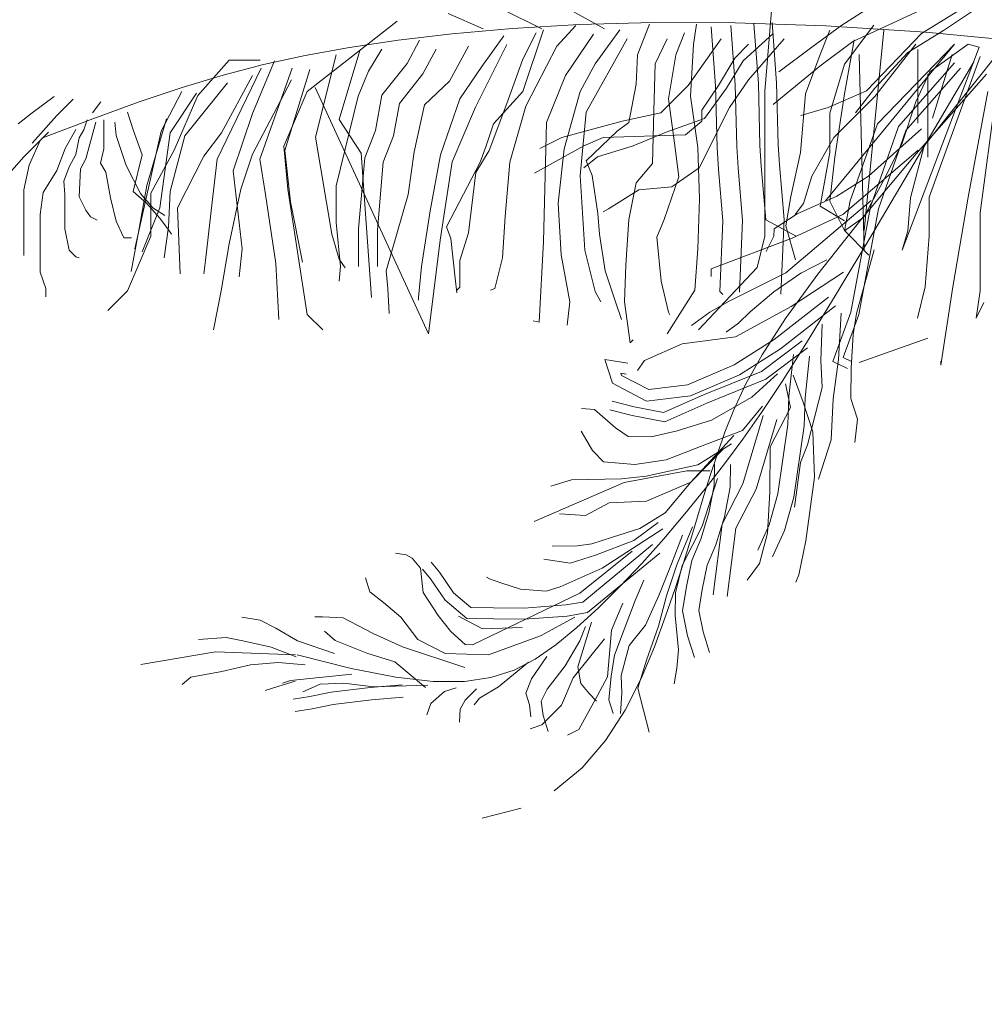
# Model space of a CAD drawing. Units: millimetres. Extents: x 595116 to 630915, y 909473 to 920225.
# Tile 82 of 134: x 629711.176 to 629720.161, y 919266.512 to 919275.684. Entities that reach past the tile are written whole.
import ezdxf

# ---------------------------------------------------------------- set-up
doc = ezdxf.new("R2010")
doc.units = ezdxf.units.MM
doc.layers.add('Dimension', color=3, linetype='Continuous', lineweight=18)
doc.layers.add('L-PLNT', color=85, linetype='Continuous', lineweight=13)
doc.styles.get("Standard").update_dxf_attribs({"font": 'arial.ttf'})
doc.dimstyles.new('ISO-25', dxfattribs={"dimtxt": 9, "dimasz": 6, "dimexe": 1.25, "dimexo": 0.625, "dimtad": 1, "dimlunit": 4, "dimtxsty": 'Standard', "dimcen": 2.5, "dimadec": 0, "dimazin": 0, "dimtfac": 1, "dimtmove": 0, "dimatfit": 3, "dimfxl": 1, "dimarcsym": 0})

# ---------------------------------------------------------------- blocks, each defined once
blk = doc.blocks.new('A$C4FB75ABC')
for p, q in [((2.1065, 2.3741), (2.087, 2.1315)), ((2.5983, 2.3508), (2.4757, 2.2759)), ((1.3881, 2.2867), (1.3008, 2.3255)), ((1.5337, 2.2867), (1.4367, 2.3352)), ((1.6891, 2.2867), (1.6017, 2.3352)), ((2.2781, 2.2963), (2.353, 2.344)), ((2.3054, 2.2555), (2.4825, 2.3372)), ((2.6119, 2.3372), (2.5302, 2.2827)), ((1.1746, 2.3061), (0.9513, 2.1315)), ((1.6258, 2.2976), (1.4598, 2.2878)), ((1.8099, 2.3026), (1.6258, 2.2976)), ((1.8004, 2.299), (1.7712, 2.2224)), ((2.0136, 2.3019), (1.8099, 2.3026)), ((1.9171, 2.299), (1.9098, 2.248)), ((2.2382, 2.2942), (2.0136, 2.3019)), ((2.0597, 2.2997), (2.0708, 2.1511)), ((2.1047, 2.3031), (2.1159, 2.1533)), ((1.3106, 2.2744), (1.1767, 2.2586)), ((1.4598, 2.2878), (1.3106, 2.2744)), ((1.5376, 2.2844), (1.4866, 2.1313)), ((1.5194, 2.2771), (1.4866, 2.2115)), ((1.6179, 2.2954), (1.5705, 2.2443)), ((1.6617, 2.2735), (1.5924, 2.1714)), ((1.7274, 2.2844), (1.6654, 2.2006)), ((1.8879, 2.2771), (1.8661, 2.2224)), ((1.9536, 2.2917), (1.9646, 2.1459)), ((2.0023, 2.2954), (2.0134, 2.1483)), ((2.1078, 2.2759), (2.0328, 2.2078)), ((2.2032, 2.2419), (2.2781, 2.2963)), ((2.2482, 2.2839), (2.2239, 2.2232)), ((2.4852, 2.2785), (2.2382, 2.2942)), ((2.3575, 2.296), (2.2846, 2.199)), ((2.3818, 2.2839), (2.3332, 1.7863)), ((2.4757, 2.2759), (2.3394, 2.1329)), ((2.5302, 2.2827), (2.4416, 2.2282)), ((2.7559, 2.2536), (2.4852, 2.2785)), ((1.1767, 2.2586), (1.0564, 2.241)), ((1.23, 2.2589), (1.1992, 2.2008)), ((1.4391, 2.2699), (1.3844, 2.1933)), ((1.7456, 2.2626), (1.6435, 2.0802)), ((1.8442, 2.2626), (1.815, 2.2006)), ((1.9783, 2.2623), (1.8966, 2.1465)), ((2.0124, 2.2146), (2.0465, 2.2487)), ((2.135, 2.2623), (2.0465, 2.1602)), ((2.2236, 2.1942), (2.3054, 2.2555)), ((2.5574, 2.2487), (2.2372, 1.8605)), ((2.3089, 2.2596), (2.2846, 2.1261)), ((2.462, 2.2487), (2.3599, 2.1193)), ((2.3667, 2.0512), (2.5574, 2.2487)), ((2.6937, 2.2623), (2.4825, 1.9967)), ((2.5915, 2.2487), (2.4961, 2.1806)), ((2.6187, 2.2419), (2.5915, 2.2487)), ((1.0564, 2.241), (0.9464, 2.2213)), ((1.0815, 2.2334), (1.0304, 2.062)), ((1.1363, 2.237), (1.1034, 2.1823)), ((1.2713, 2.237), (1.2384, 2.175)), ((1.3515, 2.2443), (1.3041, 2.1568)), ((1.4464, 2.2479), (1.3687, 2.0927)), ((1.5705, 2.2443), (1.4939, 2.0948)), ((1.9098, 2.248), (1.9025, 2.1203)), ((2.1214, 2.1806), (2.2032, 2.2419)), ((2.4416, 2.2282), (2.3599, 2.1397)), ((2.428, 1.738), (2.6187, 2.2419)), ((2.4668, 2.2354), (2.4668, 2.0533)), ((0.7572, 2.2091), (0.6795, 2.1218)), ((0.8348, 2.2091), (0.7572, 2.2091)), ((0.8699, 2.2079), (0.8151, 2.0766)), ((0.9464, 2.2213), (0.8429, 2.1986)), ((1.0231, 2.2224), (0.972, 2.0182)), ((1.1992, 2.2008), (1.1362, 2.1221)), ((1.4866, 2.2115), (1.4464, 2.1021)), ((1.6654, 2.2006), (1.6289, 2.1313)), ((1.7712, 2.2224), (1.7675, 2.1495)), ((1.815, 2.2006), (1.8113, 2.0838)), ((1.8661, 2.2224), (1.8478, 2.113)), ((1.9715, 2.1465), (2.0124, 2.2146)), ((2.0328, 2.2078), (1.992, 2.1397)), ((2.2239, 2.2232), (2.1875, 2.1261)), ((2.3211, 2.2232), (2.3332, 1.7378)), ((2.5572, 2.203), (2.4187, 2.0449)), ((2.6056, 2.2048), (2.4676, 1.9701)), ((2.6209, 2.2188), (2.4948, 1.8695)), ((2.5518, 2.2232), (2.5032, 2.0655)), ((0.837, 2.1896), (0.7276, 1.9635)), ((0.8429, 2.1986), (0.7422, 2.1723)), ((0.9137, 2.1896), (0.8334, 1.9635)), ((0.9575, 2.186), (0.8954, 1.9854)), ((1.1034, 2.1823), (1.0779, 2.1203)), ((1.2384, 2.175), (1.18, 2.1021)), ((1.3844, 2.1933), (1.3297, 2.113)), ((2.1078, 2.0989), (2.2236, 2.1942)), ((2.2846, 2.199), (2.2482, 2.0776)), ((2.5724, 2.1897), (2.4365, 2.0345)), ((2.4961, 2.1806), (2.462, 2.1057)), ((0.7422, 2.1723), (0.6405, 2.1416)), ((0.7531, 2.1531), (0.6473, 2.0218)), ((0.8151, 2.1714), (0.7385, 2.0291)), ((0.9125, 2.1606), (0.8154, 1.9763)), ((1.3041, 2.1568), (1.2421, 2.0984)), ((1.5924, 2.1714), (1.5449, 2.0547)), ((2.0465, 2.1602), (1.9988, 2.0921)), ((2.0708, 2.1511), (2.0745, 1.9975)), ((2.1159, 2.1533), (2.1196, 1.9995)), ((2.6368, 2.1742), (2.4628, 1.9766)), ((2.4911, 2.1747), (2.4911, 1.9684)), ((0.6405, 2.1416), (0.5342, 2.1057)), ((0.64, 2.1313), (0.5889, 2.0328)), ((0.6765, 2.1276), (0.6108, 2.0291)), ((0.9513, 2.1315), (0.8931, 1.9957)), ((1.2522, 1.53), (0.9707, 2.1412)), ((1.4866, 2.1313), (1.4136, 2.051)), ((1.6289, 2.1313), (1.5887, 1.989)), ((1.7675, 2.1495), (1.7493, 2.0547)), ((1.8966, 2.1465), (1.8285, 2.0784)), ((1.9306, 2.0852), (1.9715, 2.1465)), ((1.992, 2.1397), (1.9375, 2.0648)), ((1.9646, 2.1459), (1.9682, 1.9927)), ((2.0134, 2.1483), (2.017, 1.9949)), ((2.087, 2.1315), (2.087, 1.7725)), ((2.1875, 2.1261), (2.1754, 1.9805)), ((2.3394, 2.1329), (2.244, 2.0921)), ((2.2846, 2.1261), (2.2604, 1.9684)), ((2.3599, 2.1397), (2.3122, 2.0784)), ((2.6404, 2.1315), (2.5918, 1.8695)), ((0.2683, 2.0784), (0.3228, 2.1193)), ((0.3296, 2.0716), (0.3705, 2.1125)), ((0.4182, 2.0784), (0.4386, 2.1057)), ((0.5342, 2.1057), (0.4195, 2.0639)), ((0.6795, 2.1218), (0.6213, 1.986)), ((1.0779, 2.1203), (1.0231, 1.8978)), ((1.1362, 2.1221), (1.1203, 2.0346)), ((1.18, 2.1021), (1.1654, 2.0218)), ((1.3297, 2.113), (1.2822, 1.9744)), ((1.4464, 2.1021), (1.4026, 1.9854)), ((1.8478, 2.113), (1.8624, 2.0036)), ((1.9025, 2.1203), (1.9208, 1.9927)), ((2.3599, 2.1193), (2.2577, 2.0172)), ((2.462, 2.1057), (2.428, 2.0035)), ((2.6598, 2.1218), (2.6209, 1.8307)), ((0.2342, 2.0512), (0.2683, 2.0784)), ((0.505, 2.0802), (0.5196, 2.0364)), ((1.2421, 2.0984), (1.2165, 1.9817)), ((1.3687, 2.0927), (1.3105, 1.9569)), ((1.4939, 2.0948), (1.4537, 1.9562)), ((1.6435, 2.0802), (1.6289, 1.9234)), ((1.8285, 2.0784), (1.7331, 2.058)), ((1.8113, 2.0838), (1.8077, 1.9526)), ((1.9988, 2.0921), (1.9238, 1.9422)), ((1.9306, 2.058), (1.9306, 2.0852)), ((2.244, 2.0921), (2.1759, 2.0716)), ((2.2482, 2.0776), (2.2482, 1.9805)), ((0.2683, 2.0035), (0.3296, 2.0716)), ((0.4195, 2.0639), (0.2927, 2.0154)), ((0.4049, 2.0609), (0.3966, 2.0361)), ((0.427, 2.0554), (0.4021, 1.9643)), ((0.4463, 2.0609), (0.4463, 1.9892)), ((0.4739, 2.0554), (0.4767, 2.0223)), ((0.6018, 2.0636), (0.5533, 1.8986)), ((0.8151, 2.0766), (0.7677, 1.9343)), ((1.0304, 2.062), (1.0852, 1.9781)), ((1.5449, 2.0547), (1.5376, 1.7593)), ((1.7331, 2.058), (1.5832, 2.0172)), ((1.7493, 2.0547), (1.7201, 2.0328)), ((1.9375, 2.0648), (1.8421, 2.0308)), ((1.8898, 2.024), (1.9306, 2.058)), ((0.3092, 2.0308), (0.2479, 1.9695)), ((0.3773, 2.0376), (0.3501, 1.9899)), ((0.3966, 2.0361), (0.3855, 2.0168)), ((0.5196, 2.0364), (0.5415, 1.9744)), ((0.5889, 2.0328), (0.5232, 1.741)), ((0.6108, 2.0291), (0.5853, 1.8431)), ((0.7385, 2.0291), (0.6947, 1.9708)), ((1.1203, 2.0346), (1.0939, 1.9669)), ((1.4136, 2.051), (1.3953, 1.9963)), ((1.7201, 2.0328), (1.6435, 1.9598)), ((1.8421, 2.0308), (1.7603, 1.9967)), ((2.2985, 1.8605), (2.3667, 2.0512)), ((2.4756, 2.0387), (2.3438, 1.9217)), ((2.4187, 2.0449), (2.3489, 1.8456)), ((2.4365, 2.0345), (2.3686, 1.8404)), ((0.2887, 2.0103), (0.2615, 1.9491)), ((0.3855, 2.0168), (0.3773, 1.9754)), ((0.4767, 2.0223), (0.5015, 1.9478)), ((0.6473, 2.0218), (0.6108, 1.8833)), ((0.972, 2.0182), (1.0122, 1.7775)), ((1.1654, 2.0218), (1.1399, 1.9562)), ((1.5832, 2.0172), (1.5287, 1.9899)), ((1.6377, 1.9967), (1.6854, 2.0172)), ((1.6854, 2.0172), (1.8898, 2.024)), ((2.2577, 2.0172), (2.2032, 1.9218)), ((0.3501, 1.9899), (0.3296, 1.9354)), ((0.4463, 1.9892), (0.438, 1.9533)), ((0.6213, 1.986), (0.563, 1.8792)), ((0.8931, 1.9957), (0.9028, 1.8889)), ((0.8954, 1.9854), (0.91, 1.8577)), ((1.2165, 1.9817), (1.2019, 1.876)), ((1.4026, 1.9854), (1.3698, 1.9307)), ((1.3953, 1.9963), (1.3807, 1.9562)), ((1.5151, 1.9286), (1.6377, 1.9967)), ((1.5887, 1.989), (1.5741, 1.8541)), ((1.7603, 1.9967), (1.6718, 1.9695)), ((1.8624, 2.0036), (1.8734, 1.9197)), ((1.9208, 1.9927), (1.9244, 1.865)), ((1.9682, 1.9927), (1.9719, 1.938)), ((2.017, 1.9949), (2.0206, 1.9417)), ((2.0745, 1.9975), (2.0779, 1.946)), ((2.1196, 1.9995), (2.1229, 1.9495)), ((2.1754, 1.9805), (2.1511, 1.8713)), ((2.2482, 1.9805), (2.2239, 1.847)), ((2.4673, 1.986), (2.2802, 1.8264)), ((2.428, 2.0035), (2.3871, 1.9218)), ((2.4825, 1.9967), (2.4484, 1.8673)), ((0.2479, 1.9695), (0.2002, 1.915)), ((0.3773, 1.9754), (0.3607, 1.945)), ((0.4021, 1.9643), (0.3883, 1.9395)), ((0.5415, 1.9744), (0.5196, 1.8833)), ((0.6947, 1.9708), (0.629, 1.8431)), ((0.7276, 1.9635), (0.713, 1.8358)), ((0.8154, 1.9763), (0.7863, 1.8889)), ((0.8334, 1.9635), (0.848, 1.876)), ((1.0939, 1.9669), (1.0786, 1.7905)), ((1.0852, 1.9781), (1.1107, 1.6207)), ((1.1399, 1.9562), (1.1253, 1.7884)), ((1.2822, 1.9744), (1.2567, 1.8358)), ((1.3105, 1.9569), (1.2814, 1.7628)), ((1.3807, 1.9562), (1.2968, 1.7957)), ((1.4537, 1.9562), (1.4428, 1.8213)), ((1.6718, 1.9695), (1.6377, 1.9422)), ((1.6435, 1.9598), (1.6581, 1.9234)), ((2.2604, 1.9684), (2.2482, 1.8591)), ((2.4628, 1.9766), (2.3249, 1.8127)), ((2.4676, 1.9701), (2.3552, 1.7802)), ((0.2615, 1.9491), (0.2479, 1.8878)), ((0.3296, 1.9354), (0.2956, 1.881)), ((0.3607, 1.945), (0.3469, 1.9091)), ((0.3883, 1.9395), (0.3855, 1.8705)), ((0.438, 1.9533), (0.4518, 1.9312)), ((0.4518, 1.9312), (0.4629, 1.8677)), ((0.5015, 1.9478), (0.5374, 1.8788)), ((0.7677, 1.9343), (0.7896, 1.741)), ((1.3698, 1.9307), (1.3515, 1.7811)), ((1.8077, 1.9526), (1.7675, 1.9051)), ((1.9238, 1.9422), (1.8557, 1.8946)), ((1.9719, 1.938), (1.9828, 1.8103)), ((2.0206, 1.9417), (2.0317, 1.8114)), ((2.0779, 1.946), (2.0893, 1.8127)), ((2.1229, 1.9495), (2.1345, 1.8136)), ((0.3469, 1.9091), (0.3497, 1.876)), ((1.6289, 1.9234), (1.6398, 1.7374)), ((1.6581, 1.9234), (1.6727, 1.8285)), ((1.8734, 1.9197), (1.8369, 1.814)), ((2.2032, 1.9218), (2.1827, 1.8537)), ((2.3438, 1.9217), (2.2657, 1.8718)), ((2.3871, 1.9218), (2.3326, 1.8197)), ((0.2479, 1.8878), (0.2479, 1.8061)), ((0.5196, 1.8833), (0.5524, 1.8541)), ((0.5533, 1.8986), (0.5339, 1.7919)), ((0.6108, 1.8833), (0.6072, 1.7957)), ((0.7863, 1.8889), (0.7572, 1.7531)), ((0.9028, 1.8889), (0.9513, 1.5785)), ((1.0231, 1.8978), (1.0231, 1.8067)), ((1.7739, 1.8878), (1.699, 1.8401)), ((1.7675, 1.9051), (1.7493, 1.814)), ((1.8557, 1.8946), (1.7739, 1.8878)), ((0.2956, 1.881), (0.2887, 1.8265)), ((0.3497, 1.876), (0.3497, 1.8512)), ((0.3855, 1.8705), (0.4021, 1.8374)), ((0.4629, 1.8677), (0.4767, 1.8098)), ((0.5374, 1.8788), (0.5678, 1.8429)), ((0.563, 1.8792), (0.563, 1.7725)), ((0.848, 1.876), (0.8735, 1.7045)), ((0.91, 1.8577), (0.9392, 1.7082)), ((1.2019, 1.876), (1.1472, 1.6863)), ((1.9244, 1.865), (1.9208, 1.741)), ((2.3505, 1.8613), (2.1386, 1.6813)), ((2.1511, 1.8713), (2.1389, 1.7985)), ((2.2657, 1.8718), (2.167, 1.8279)), ((2.2482, 1.8591), (2.2846, 1.7863)), ((2.2849, 1.7856), (2.2985, 1.8605)), ((2.4484, 1.8673), (2.4416, 1.7856)), ((2.4948, 1.8695), (2.4948, 1.7725)), ((2.5918, 1.8695), (2.553, 1.6464)), ((0.3497, 1.8512), (0.3497, 1.7904)), ((0.4021, 1.8374), (0.4132, 1.8208)), ((0.5853, 1.8431), (0.5415, 1.7337)), ((0.5524, 1.8541), (0.5853, 1.8176)), ((0.5678, 1.8429), (0.5982, 1.8236)), ((0.629, 1.8431), (0.6363, 1.679)), ((0.713, 1.8358), (0.6984, 1.7118)), ((1.2567, 1.8358), (1.2348, 1.6973)), ((1.5741, 1.8541), (1.5814, 1.7264)), ((1.699, 1.8401), (1.6854, 1.8333)), ((2.1827, 1.8537), (2.1623, 1.8265)), ((2.2239, 1.847), (2.2846, 1.8106)), ((2.3489, 1.8456), (2.3004, 1.5838)), ((2.3686, 1.8404), (2.32, 1.5785)), ((0.2887, 1.8265), (0.2887, 1.7516)), ((0.4132, 1.8208), (0.4297, 1.8125)), ((0.4767, 1.8098), (0.496, 1.7684)), ((0.5853, 1.8176), (0.6072, 1.7884)), ((1.4428, 1.8213), (1.4355, 1.7191)), ((1.6727, 1.8285), (1.6763, 1.7775)), ((1.7493, 1.814), (1.742, 1.7009)), ((1.8369, 1.814), (1.8186, 1.7702)), ((1.9828, 1.8103), (1.9755, 1.6352)), ((2.0317, 1.8114), (2.0243, 1.6332)), ((2.0893, 1.8127), (2.1647, 1.7725)), ((2.167, 1.8279), (2.1099, 1.791)), ((2.1345, 1.8136), (2.1268, 1.6289)), ((2.2802, 1.8264), (2.1549, 1.7678)), ((2.3249, 1.8127), (2.2184, 1.678)), ((2.3326, 1.8197), (2.2849, 1.7856)), ((2.6209, 1.8307), (2.6209, 1.6367)), ((0.2479, 1.8061), (0.2479, 1.7448)), ((0.3497, 1.7904), (0.3607, 1.738)), ((0.5339, 1.7919), (0.5145, 1.6852)), ((0.6072, 1.7957), (0.5962, 1.7191)), ((0.6072, 1.7884), (0.6144, 1.7775)), ((1.0231, 1.8067), (1.0341, 1.6973)), ((1.0786, 1.7905), (1.0786, 1.6973)), ((1.1253, 1.7884), (1.1253, 1.7665)), ((1.2968, 1.7957), (1.3078, 1.7665)), ((2.1099, 1.791), (2.1096, 1.7722)), ((2.1389, 1.7985), (2.1632, 1.7135)), ((2.2846, 1.7863), (2.3453, 1.7256)), ((2.4416, 1.7856), (2.428, 1.738)), ((0.496, 1.7684), (0.5153, 1.7684)), ((0.563, 1.7725), (0.5048, 1.6367)), ((1.0122, 1.7775), (1.0304, 1.7155)), ((1.1253, 1.7665), (1.1253, 1.7301)), ((1.2814, 1.7628), (1.2522, 1.53)), ((1.3078, 1.7665), (1.3187, 1.6681)), ((1.3515, 1.7811), (1.3297, 1.7118)), ((1.6763, 1.7775), (1.6909, 1.6863)), ((1.8186, 1.7702), (1.8296, 1.6608)), ((2.1549, 1.7678), (1.9538, 1.6913)), ((2.087, 1.7725), (2.0676, 1.6949)), ((2.1096, 1.7722), (2.0903, 1.7347)), ((2.3552, 1.7802), (2.2641, 1.6283)), ((2.4948, 1.7725), (2.485, 1.6464)), ((0.2479, 1.7448), (0.2479, 1.7243)), ((0.2887, 1.7516), (0.2887, 1.6835)), ((0.3607, 1.738), (0.3773, 1.7214)), ((0.7572, 1.7531), (0.7377, 1.6367)), ((0.7896, 1.741), (0.7823, 1.6717)), ((1.5376, 1.7593), (1.5267, 1.5587)), ((1.6398, 1.7374), (1.6654, 1.6352)), ((1.9208, 1.741), (1.9135, 1.6389)), ((2.3582, 1.7386), (2.3145, 1.5808)), ((0.3773, 1.7214), (0.3855, 1.7187)), ((0.6984, 1.7118), (0.6947, 1.679)), ((1.0304, 1.7155), (1.045, 1.6936)), ((1.1253, 1.7301), (1.1253, 1.6973)), ((1.3297, 1.7118), (1.3297, 1.6462)), ((1.4355, 1.7191), (1.4172, 1.6425)), ((1.5814, 1.7264), (1.6033, 1.6097)), ((2.2409, 1.7138), (2.1763, 1.6807)), ((0.8735, 1.7045), (0.8808, 1.566)), ((1.0341, 1.6973), (1.0304, 1.6608)), ((1.1472, 1.6863), (1.1509, 1.6425)), ((1.2348, 1.6973), (1.2275, 1.6207)), ((1.6909, 1.6863), (1.7164, 1.6097)), ((1.742, 1.7009), (1.7383, 1.6097)), ((2.0676, 1.6949), (1.922, 1.5397)), ((1.9538, 1.6913), (1.9536, 1.6725)), ((0.2887, 1.6835), (0.3024, 1.6426)), ((1.3187, 1.6681), (1.3224, 1.6316)), ((2.1386, 1.6813), (1.998, 1.6115)), ((2.1763, 1.6807), (2.1096, 1.6345)), ((2.2184, 1.678), (2.1385, 1.568)), ((2.2819, 1.6831), (2.1525, 1.5981)), ((0.3024, 1.6426), (0.3024, 1.6222)), ((1.1509, 1.6425), (1.1545, 1.5805)), ((1.3297, 1.6462), (1.3224, 1.6389)), ((1.4172, 1.6425), (1.4063, 1.6389)), ((1.8296, 1.6608), (1.8478, 1.5842)), ((1.9135, 1.6389), (1.8444, 1.53)), ((2.485, 1.6464), (2.4656, 1.5688)), ((2.553, 1.6464), (2.5239, 1.4523)), ((0.5048, 1.6367), (0.4562, 1.5882)), ((0.7377, 1.6367), (0.7183, 1.5397)), ((1.2275, 1.6207), (1.2275, 1.6134)), ((1.6654, 1.6352), (1.68, 1.6097)), ((1.9755, 1.6352), (1.9828, 1.628)), ((2.1096, 1.6345), (2.0504, 1.5844)), ((2.2452, 1.6213), (2.1098, 1.5157)), ((2.2641, 1.6283), (2.1904, 1.5079)), ((2.6209, 1.6367), (2.6112, 1.5688)), ((1.6033, 1.6097), (1.596, 1.5514)), ((1.7164, 1.6097), (1.731, 1.566)), ((1.7383, 1.6097), (1.7529, 1.5076)), ((1.998, 1.6115), (1.9504, 1.5839)), ((2.1525, 1.5981), (2.0137, 1.5227)), ((2.2623, 1.5995), (2.1258, 1.493)), ((2.6112, 1.5688), (2.6307, 1.6076)), ((0.9513, 1.5785), (0.9901, 1.5397)), ((1.8478, 1.5842), (1.8515, 1.5769)), ((1.9504, 1.5839), (1.9047, 1.5506)), ((2.0504, 1.5844), (2.0217, 1.5565)), ((2.1385, 1.568), (2.0803, 1.4783)), ((2.3004, 1.5838), (2.256, 1.4617)), ((2.2767, 1.5813), (2.2695, 1.4664)), ((2.32, 1.5785), (2.2812, 1.4717)), ((2.3145, 1.5808), (2.3062, 1.5281)), ((1.5267, 1.5587), (1.5121, 1.5623)), ((2.0217, 1.5565), (1.9912, 1.5343)), ((2.2292, 1.5537), (2.2261, 1.4651)), ((2.0137, 1.5227), (1.8814, 1.5056)), ((2.1098, 1.5157), (2.0109, 1.453)), ((2.3062, 1.5281), (2.3013, 1.4452)), ((2.4911, 1.5193), (2.3211, 1.4586)), ((1.7529, 1.5076), (1.7602, 1.5149)), ((1.8814, 1.5056), (1.7884, 1.4636)), ((2.1258, 1.493), (2.0238, 1.4284)), ((2.1796, 1.5129), (2.0785, 1.437)), ((2.1927, 1.4954), (2.0894, 1.4177)), ((2.1904, 1.5079), (2.1298, 1.4122)), ((1.7084, 1.4073), (1.6895, 1.4666)), ((1.6895, 1.4666), (1.747, 1.4576)), ((2.0803, 1.4783), (2.039, 1.4043)), ((2.1578, 1.4791), (2.1468, 1.3743)), ((2.1979, 1.4749), (2.187, 1.3714)), ((2.2695, 1.4664), (2.2568, 1.3685)), ((2.2812, 1.4717), (2.3006, 1.462)), ((1.7884, 1.4636), (1.7711, 1.4393)), ((2.0109, 1.453), (1.8951, 1.4036)), ((2.2261, 1.4651), (2.2289, 1.3972)), ((2.256, 1.4617), (2.2916, 1.4439)), ((2.3013, 1.4452), (2.3002, 1.3698)), ((2.5239, 1.4523), (2.5239, 1.462)), ((1.7313, 1.4266), (1.7295, 1.4323)), ((1.7295, 1.4323), (1.7427, 1.4302)), ((1.7987, 1.3918), (1.7313, 1.4266)), ((2.0238, 1.4284), (1.9024, 1.3766)), ((2.0785, 1.437), (1.9344, 1.3786)), ((2.0894, 1.4177), (1.9429, 1.3584)), ((2.1181, 1.4308), (2.055, 1.3732)), ((2.1569, 1.4277), (2.1816, 1.3609)), ((1.7936, 1.3632), (1.7084, 1.4073)), ((1.8951, 1.4036), (1.7987, 1.3918)), ((2.039, 1.4043), (2.0098, 1.3416)), ((2.1298, 1.4122), (2.0784, 1.3347)), ((2.1385, 1.406), (2.1509, 1.3473)), ((2.2289, 1.3972), (2.1929, 1.2544)), ((1.9024, 1.3766), (1.7936, 1.3632)), ((1.9344, 1.3786), (1.8357, 1.3347)), ((2.055, 1.3732), (1.9542, 1.3161)), ((2.1468, 1.3743), (2.1439, 1.3053)), ((2.187, 1.3714), (2.1842, 1.3016)), ((2.2568, 1.3685), (2.2516, 1.2668)), ((2.3002, 1.3698), (2.3165, 1.3187)), ((1.6641, 1.3427), (1.6321, 1.345)), ((1.7623, 1.3489), (1.7078, 1.3628)), ((1.8357, 1.3347), (1.7623, 1.3489)), ((1.9429, 1.3584), (1.8383, 1.3119)), ((2.0811, 1.3502), (2.0312, 1.2905)), ((2.1509, 1.3473), (2.1005, 1.25)), ((2.1816, 1.3609), (2.2062, 1.287)), ((1.7163, 1.2967), (1.6641, 1.3427)), ((1.7575, 1.3275), (1.7024, 1.3416)), ((1.8383, 1.3119), (1.7575, 1.3275)), ((2.0098, 1.3416), (1.9878, 1.2857)), ((2.0784, 1.3347), (2.0319, 1.2687)), ((2.0829, 1.3276), (2.0324, 1.158)), ((1.7481, 1.2755), (1.7163, 1.2967)), ((1.9542, 1.3161), (1.869, 1.289)), ((2.1165, 1.3176), (2.065, 1.1449)), ((2.1439, 1.3053), (2.1195, 1.1332)), ((2.1842, 1.3016), (2.1591, 1.1247)), ((2.3165, 1.3187), (2.31, 1.2603)), ((1.6589, 1.2409), (1.6313, 1.2885)), ((1.8046, 1.2748), (1.7481, 1.2755)), ((1.869, 1.289), (1.8046, 1.2748)), ((2.0103, 1.2776), (1.903, 1.1622)), ((2.0312, 1.2905), (1.9421, 1.2559)), ((1.9878, 1.2857), (1.9691, 1.2327)), ((2.2062, 1.287), (2.2097, 1.1745)), ((1.9421, 1.2559), (1.8416, 1.2177)), ((2.0043, 1.257), (1.9206, 1.2053)), ((2.0319, 1.2687), (1.9864, 1.2075)), ((2.1005, 1.25), (2.0989, 1.1369)), ((2.1929, 1.2544), (2.1754, 1.2112)), ((2.2516, 1.2668), (2.22, 1.1691)), ((1.6868, 1.2123), (1.6589, 1.2409)), ((1.9834, 1.244), (1.903, 1.1622)), ((1.9691, 1.2327), (1.952, 1.1808)), ((1.7641, 1.2056), (1.6868, 1.2123)), ((1.8416, 1.2177), (1.7641, 1.2056)), ((1.9206, 1.2053), (1.792, 1.1769)), ((1.9864, 1.2075), (1.9386, 1.1458)), ((1.9621, 1.2066), (1.9614, 1.1536)), ((2.0017, 1.2061), (2.001, 1.1495)), ((2.1754, 1.2112), (2.1606, 1.1002)), ((1.792, 1.1769), (1.7315, 1.1702)), ((1.7376, 1.1613), (1.8929, 1.1904)), ((1.8929, 1.1904), (1.9511, 1.1904)), ((1.952, 1.1808), (1.9358, 1.129)), ((2.2097, 1.1745), (2.1886, 1.0162)), ((1.5143, 1.0642), (1.7376, 1.1613)), ((1.607, 1.1681), (1.5558, 1.1518)), ((1.7315, 1.1702), (1.607, 1.1681)), ((1.903, 1.1622), (1.793, 1.1147)), ((1.903, 1.1622), (1.8397, 1.0857)), ((1.9692, 1.1707), (1.9317, 1.0524)), ((1.9614, 1.1536), (1.9482, 1.0859)), ((2.0324, 1.158), (1.9806, 1.0581)), ((2.001, 1.1495), (1.9867, 1.0762)), ((1.9386, 1.1458), (1.8882, 1.0835)), ((1.9358, 1.129), (1.9198, 1.076)), ((2.065, 1.1449), (2.0146, 1.0475)), ((2.0989, 1.1369), (2.0937, 1.0351)), ((2.1195, 1.1332), (2.0972, 1.056)), ((2.1591, 1.1247), (2.1353, 1.0421)), ((1.7005, 1.1103), (1.6416, 1.079)), ((1.793, 1.1147), (1.7005, 1.1103)), ((1.6416, 1.079), (1.5775, 1.0837)), ((1.8397, 1.0857), (1.7769, 1.047)), ((1.8882, 1.0835), (1.8359, 1.0215)), ((1.9198, 1.076), (1.903, 1.0206)), ((1.9482, 1.0859), (1.9278, 1.0204)), ((1.9867, 1.0762), (1.965, 1.0067)), ((1.8224, 1.0615), (1.7614, 1.017)), ((1.9071, 1.0509), (1.8681, 0.9571)), ((1.9317, 1.0524), (1.8813, 0.9551)), ((1.9806, 1.0581), (1.9586, 0.8825)), ((2.0972, 1.056), (2.0692, 0.9929)), ((1.8335, 1.0462), (1.6831, 0.9483)), ((1.7769, 1.047), (1.7087, 1.0253)), ((1.8823, 1.0305), (1.8549, 0.9592)), ((2.0146, 1.0475), (2.004, 0.9628)), ((2.0937, 1.0351), (2.0738, 0.96)), ((2.1353, 1.0421), (2.1061, 0.9765)), ((1.6216, 1.0039), (1.5594, 1.0028)), ((1.6576, 1.009), (1.6216, 1.0039)), ((1.8084, 1.007), (1.6348, 0.8642)), ((1.7087, 1.0253), (1.6576, 1.009)), ((1.7614, 1.017), (1.6666, 0.9806)), ((1.8359, 1.0215), (1.7823, 0.9612)), ((1.903, 1.0206), (1.8847, 0.9618)), ((1.9278, 1.0204), (1.9055, 0.9679)), ((1.965, 1.0067), (1.9435, 0.9561)), ((2.1886, 1.0162), (2.171, 0.9318)), ((1.1969, 0.9814), (1.1705, 0.9855)), ((1.2119, 0.9737), (1.1969, 0.9814)), ((1.6666, 0.9806), (1.6041, 0.9607)), ((1.7573, 0.9907), (1.6276, 0.8869)), ((1.8259, 0.9857), (1.6466, 0.8382)), ((1.2323, 0.9489), (1.2119, 0.9737)), ((1.2793, 0.9388), (1.2589, 0.9636)), ((1.6041, 0.9607), (1.5382, 0.9711)), ((1.7823, 0.9612), (1.7281, 0.9036)), ((1.8549, 0.9592), (1.8236, 0.8804)), ((1.8681, 0.9571), (1.8425, 0.8802)), ((1.8847, 0.9618), (1.8642, 0.8983)), ((1.8813, 0.9551), (1.8652, 0.8874)), ((1.9055, 0.9679), (1.8924, 0.9029)), ((1.9435, 0.9561), (1.9314, 0.8959)), ((2.004, 0.9628), (1.9934, 0.8781)), ((2.0738, 0.96), (2.043, 0.9189)), ((1.239, 0.8884), (1.2323, 0.9489)), ((1.2572, 0.9222), (1.2376, 0.9461)), ((1.3144, 0.8874), (1.2793, 0.9388)), ((1.6831, 0.9483), (1.5787, 0.9026)), ((2.171, 0.9318), (2.164, 0.9142)), ((1.107, 0.8902), (1.0961, 0.9243)), ((1.2938, 0.8688), (1.2572, 0.9222)), ((1.4036, 0.922), (1.3961, 0.9259)), ((1.4317, 0.9122), (1.4036, 0.922)), ((1.4805, 0.8964), (1.4317, 0.9122)), ((1.7864, 0.9186), (1.765, 0.868)), ((1.1405, 0.8634), (1.107, 0.8902)), ((1.2759, 0.8314), (1.239, 0.8884)), ((1.3573, 0.851), (1.3144, 0.8874)), ((1.6276, 0.8869), (1.3617, 0.7585)), ((1.5446, 0.8918), (1.4805, 0.8964)), ((1.5787, 0.9026), (1.5446, 0.8918)), ((1.7281, 0.9036), (1.6739, 0.8498)), ((1.8236, 0.8804), (1.7906, 0.8073)), ((1.8425, 0.8802), (1.8226, 0.805)), ((1.8642, 0.8983), (1.8405, 0.829)), ((1.8652, 0.8874), (1.8644, 0.8308)), ((1.8924, 0.9029), (1.8829, 0.8424)), ((1.9314, 0.8959), (1.9231, 0.8432)), ((1.1834, 0.827), (1.1405, 0.8634)), ((1.347, 0.8236), (1.2938, 0.8688)), ((1.5932, 0.8572), (1.4893, 0.8492)), ((1.6348, 0.8642), (1.5932, 0.8572)), ((1.7347, 0.8614), (1.7065, 0.7946)), ((1.765, 0.868), (1.7376, 0.7967)), ((1.3074, 0.7913), (1.2759, 0.8314)), ((1.4139, 0.8502), (1.3573, 0.851)), ((1.4893, 0.8492), (1.4139, 0.8502)), ((1.6466, 0.8382), (1.5965, 0.8298)), ((1.6739, 0.8498), (1.6204, 0.8011)), ((1.8829, 0.8424), (1.8952, 0.7804)), ((1.9231, 0.8432), (1.9337, 0.7903)), ((0.8346, 0.8198), (0.7888, 0.827)), ((0.8736, 0.7996), (0.8346, 0.8198)), ((0.9891, 0.8277), (0.9703, 0.828)), ((1.04, 0.8252), (0.9891, 0.8277)), ((1.1149, 0.7864), (1.04, 0.8252)), ((1.226, 0.7717), (1.1834, 0.827)), ((1.3863, 0.7981), (1.3265, 0.8298)), ((1.4135, 0.8227), (1.347, 0.8236)), ((1.4902, 0.8216), (1.4135, 0.8227)), ((1.5965, 0.8298), (1.4902, 0.8216)), ((1.6154, 0.8267), (1.5299, 0.7807)), ((1.6567, 0.8148), (1.6231, 0.704)), ((1.7906, 0.8073), (1.7502, 0.757)), ((1.8405, 0.829), (1.8129, 0.7535)), ((1.8644, 0.8308), (1.8727, 0.7459)), ((0.9273, 0.7678), (0.8736, 0.7996)), ((1.0204, 0.7689), (0.9943, 0.7918)), ((1.188, 0.7534), (1.1149, 0.7864)), ((1.3428, 0.7588), (1.3074, 0.7913)), ((1.4848, 0.8016), (1.3863, 0.7981)), ((1.6204, 0.8011), (1.5682, 0.7585)), ((1.6415, 0.8037), (1.6278, 0.7681)), ((1.7065, 0.7946), (1.696, 0.6785)), ((1.7376, 0.7967), (1.7141, 0.733)), ((1.8226, 0.805), (1.7931, 0.7206)), ((1.9337, 0.7903), (1.9499, 0.7392)), ((0.7503, 0.7767), (0.6814, 0.7711)), ((0.7912, 0.768), (0.7503, 0.7767)), ((0.8615, 0.7523), (0.7912, 0.768)), ((1.0187, 0.737), (0.9273, 0.7678)), ((1.0992, 0.7376), (1.0204, 0.7689)), ((1.2935, 0.7368), (1.226, 0.7717)), ((1.3617, 0.7585), (1.3428, 0.7588)), ((1.5299, 0.7807), (1.4009, 0.7335)), ((1.5682, 0.7585), (1.5172, 0.7231)), ((1.6278, 0.7681), (1.5911, 0.7064)), ((1.6891, 0.7732), (1.6114, 0.6762)), ((1.8952, 0.7804), (1.9122, 0.7271)), ((0.7236, 0.7411), (0.5379, 0.7092)), ((0.9219, 0.7334), (0.7236, 0.7411)), ((0.9235, 0.7285), (0.8615, 0.7523)), ((1.0599, 0.6997), (0.9265, 0.7333)), ((1.1687, 0.7159), (1.0992, 0.7376)), ((1.342, 0.7022), (1.188, 0.7534)), ((1.4009, 0.7335), (1.2935, 0.7368)), ((1.7502, 0.757), (1.7303, 0.6818)), ((1.8129, 0.7535), (1.7799, 0.6746)), ((1.8727, 0.7459), (1.8683, 0.7007)), ((0.8101, 0.7087), (0.7393, 0.6917)), ((0.879, 0.7143), (0.8101, 0.7087)), ((0.9462, 0.7085), (0.879, 0.7143)), ((1.2451, 0.6526), (1.1687, 0.7159)), ((1.5006, 0.7151), (1.4262, 0.6539)), ((1.5172, 0.7231), (1.4647, 0.6957)), ((1.5461, 0.7296), (1.5076, 0.6736)), ((1.7141, 0.733), (1.7058, 0.6803)), ((1.7931, 0.7206), (1.7714, 0.6511)), ((0.7393, 0.6917), (0.6621, 0.678)), ((1.0623, 0.6856), (0.9095, 0.6697)), ((1.1712, 0.6779), (1.0599, 0.6997)), ((1.4647, 0.6957), (1.4072, 0.6768)), ((1.5911, 0.7064), (1.5469, 0.6485)), ((1.6231, 0.704), (1.6301, 0.6625)), ((1.8683, 0.7007), (1.8621, 0.6612)), ((0.6621, 0.678), (0.6405, 0.6602)), ((0.9209, 0.6684), (0.8811, 0.6557)), ((0.9095, 0.6697), (0.8898, 0.6634)), ((0.9832, 0.6605), (0.9403, 0.6414)), ((1.0423, 0.6629), (0.9832, 0.6605)), ((1.1159, 0.6537), (1.0423, 0.6629)), ((1.2639, 0.6673), (1.1712, 0.6779)), ((1.3414, 0.6671), (1.2639, 0.6673)), ((1.4072, 0.6768), (1.3414, 0.6671)), ((1.5076, 0.6736), (1.4939, 0.6379)), ((1.6114, 0.6762), (1.5823, 0.6082)), ((1.6301, 0.6625), (1.6505, 0.6377)), ((1.696, 0.6785), (1.6713, 0.6328)), ((1.7058, 0.6803), (1.6993, 0.6219)), ((1.7303, 0.6818), (1.7316, 0.6384)), ((1.7799, 0.6746), (1.74, 0.5958)), ((0.8811, 0.6557), (0.847, 0.6449)), ((1.011, 0.6408), (0.9581, 0.6302)), ((1.1074, 0.6526), (1.011, 0.6408)), ((1.1867, 0.6591), (1.1074, 0.6526)), ((1.2504, 0.6584), (1.1159, 0.6537)), ((1.2921, 0.6426), (1.2578, 0.6129)), ((1.3206, 0.6516), (1.2921, 0.6426)), ((1.3714, 0.649), (1.3428, 0.6211)), ((1.4262, 0.6539), (1.3787, 0.6263)), ((1.4939, 0.6379), (1.5029, 0.6095)), ((1.5469, 0.6485), (1.5314, 0.6186)), ((1.6505, 0.6377), (1.6691, 0.6186)), ((1.7316, 0.6384), (1.729, 0.5876)), ((1.7714, 0.6511), (1.8, 0.5413)), ((0.9581, 0.6302), (0.9165, 0.6232)), ((1.1106, 0.6216), (1.016, 0.61)), ((1.1893, 0.628), (1.1106, 0.6216)), ((1.2578, 0.6129), (1.2479, 0.5847)), ((1.3428, 0.6211), (1.3311, 0.5987)), ((1.3787, 0.6263), (1.3652, 0.6095)), ((1.5314, 0.6186), (1.5365, 0.5827)), ((1.6713, 0.6328), (1.6256, 0.5484)), ((1.6993, 0.6219), (1.7101, 0.5878)), ((0.9632, 0.5994), (0.9216, 0.5925)), ((1.016, 0.61), (0.9632, 0.5994)), ((1.3311, 0.5987), (1.3288, 0.5666)), ((1.5029, 0.6095), (1.5063, 0.5793)), ((1.5823, 0.6082), (1.5337, 0.5597)), ((1.74, 0.5958), (1.6917, 0.5207)), ((1.5365, 0.5827), (1.5492, 0.5429)), ((1.5337, 0.5597), (1.5046, 0.55)), ((1.6256, 0.5484), (1.5974, 0.5343)), ((1.6917, 0.5207), (1.6336, 0.4527)), ((1.6336, 0.4527), (1.5642, 0.3956)), ((1.4819, 0.3527), (1.3853, 0.3277))]:
    blk.add_line(p, q)
blk = doc.blocks.new('*D216')
at = {"layer": 'Defpoints', "color": 0, "transparency": 16777216}
for p in [(629743.5408, 919411.9276), (629505.0408, 919411.8279), (629743.5408, 918832.3776)]:
    blk.add_point(p, dxfattribs=at)
at = {"layer": 'Dimension', "color": 0, "lineweight": -2, "transparency": 16777216}
for p, q in [((629743.5408, 919411.3026), (629743.5408, 918831.1276)), ((629505.0408, 919411.2029), (629505.0408, 918831.1276)), ((629511.0408, 918832.3776), (629737.5408, 918832.3776))]:
    blk.add_line(p, q, dxfattribs=at)
at = {"layer": 'Dimension', "color": 0, "transparency": 16777216}
for points in [[(629511.0408, 918833.3776), (629511.0408, 918831.3776), (629505.0408, 918832.3776)], [(629737.5408, 918833.3776), (629737.5408, 918831.3776), (629743.5408, 918832.3776)]]:
    blk.add_solid(points, dxfattribs=at)
at = {"layer": 'Dimension', "color": 0, "transparency": 16777216, "insert": (629624.2908, 918837.656), "char_height": 9, "attachment_point": 5}
blk.add_mtext('19\'-10 1/2"', dxfattribs=at)

msp = doc.modelspace()

# ---------------------------------------------------------------- block references
at = {"layer": 'L-PLNT', "xscale": 3.753413438031968, "yscale": 3.753413438031968, "zscale": 3.753413438031968}
msp.add_blockref('A$C4FB75ABC', (629710.2837, 919267.0144), dxfattribs=at)

# ---------------------------------------------------------------- dimensions: what is measured, and where the dimension line sits
at = {"layer": 'Dimension'}
dim = msp.add_linear_dim(base=(629743.5408, 918832.3776), p1=(629505.0408, 919411.8279), p2=(629743.5408, 919411.9276), dimstyle='ISO-25', override={"dimdec": 1, "dimlfac": 1, "dimrnd": 0, "dimzin": 1, "dimdsep": 46, "dimlunit": 4, "dimfrac": 2}, dxfattribs=at)
dim.commit()
dim.dimension.update_dxf_attribs({"geometry": '*D216', "text_midpoint": (629624.2908, 918837.656)})

doc.saveas('drawing.dxf')
